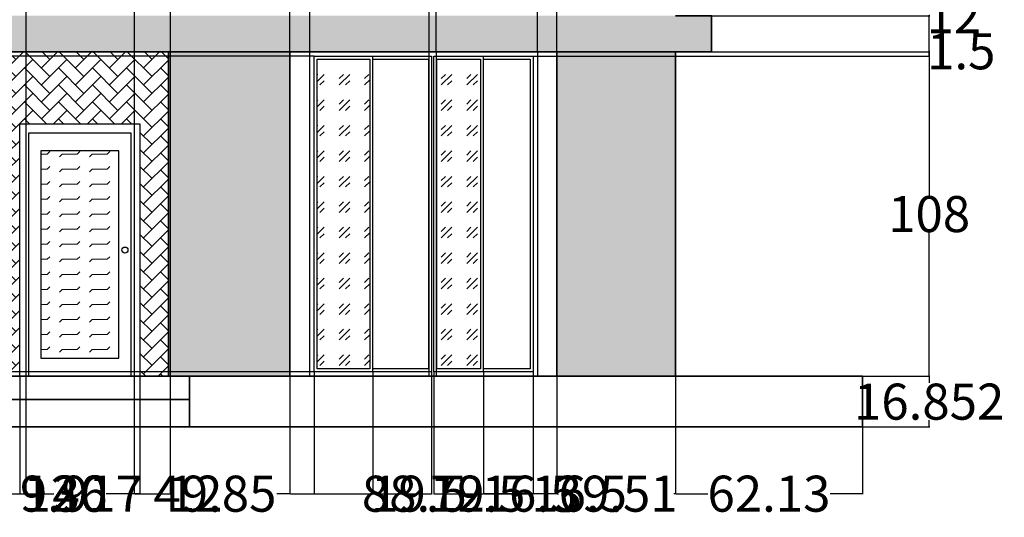
# Model space of a CAD drawing. Units: inches. Extents: x -73 to 458, y -161 to 332.
# Tile 2 of 6: x 106 to 433, y -161 to 5. Entities that reach past the tile are written whole.
import ezdxf

# ---------------------------------------------------------------- set-up
doc = ezdxf.new("R2010")
doc.units = ezdxf.units.IN
doc.header["$MEASUREMENT"] = 0
for name, color, linetype, lineweight in [('A-ANNO-DIMS', 2, 'Continuous', 18), ('A-DOOR', 4, 'Continuous', 25), ('A-ELEV', 7, 'Continuous', 35), ('A-ELEV-PATT', 8, 'Continuous', 13), ('A-GLAZ', 3, 'Continuous', 25), ('A-GLAZ-PATT', 8, 'Continuous', 13)]:
    doc.layers.add(name, color=color, linetype=linetype, lineweight=lineweight)
doc.styles.get("Standard").update_dxf_attribs({"font": 'arial.ttf'})
doc.dimstyles.get("Standard").update_dxf_attribs({"dimtxt": 12, "dimasz": 0.18, "dimexe": 0.18, "dimexo": 0.0625, "dimgap": 0.09, "dimtad": 0, "dimtih": 1, "dimtoh": 1, "dimdec": 0, "dimzin": 0, "dimdsep": 46, "dimlunit": 3, "dimtxsty": 'Standard', "dimcen": 0.09, "dimadec": 0, "dimazin": 0, "dimtfac": 1, "dimtdec": 0, "dimtofl": 0, "dimtmove": 0, "dimatfit": 3, "dimfxl": 1, "dimtolj": 1, "dimtzin": 0, "dimarcsym": 0})

# ---------------------------------------------------------------- blocks, each defined once
blk = doc.blocks.new('*U3')
blk.add_lwpolyline([(3.12, 0.01), (0.12, 0.01), (0.12, 84.01), (40.12, 84.01), (40.12, 0.01), (37.12, 0.01)])
for points in [[(37.12, 80.99), (37.12, 0.01), (3.12, 0.01), (3.12, 80.99)], [(33.12, 6.01), (33.12, 74.99), (7.12, 74.99), (7.12, 6.01)]]:
    blk.add_lwpolyline(points, close=True)
blk.add_circle((35.12, 42.01), 1)
blk = doc.blocks.new('*D11')
at = {"layer": 'A-ANNO-DIMS', "color": 0, "lineweight": -2, "transparency": 16777216}
for p, q in [((96, -114), (96, -153.17)), ((105.91, -113.98), (105.91, -153.17)), ((96.18, -152.99), (105.73, -152.99)), ((105.91, -152.99), (106.09, -152.99))]:
    blk.add_line(p, q, dxfattribs=at)
at = {"layer": 'A-ANNO-DIMS', "color": 0, "transparency": 16777216}
for points in [[(96.18, -152.96), (96.18, -153.02), (96, -152.99)], [(105.73, -152.96), (105.73, -153.02), (105.91, -152.99)]]:
    blk.add_solid(points, dxfattribs=at)
at = {"layer": 'Defpoints', "color": 0, "transparency": 16777216}
for p in [(96, -113.93), (105.91, -113.92), (105.91, -152.99)]:
    blk.add_point(p, dxfattribs=at)
at = {"layer": 'A-ANNO-DIMS', "color": 0, "transparency": 16777216, "insert": (126.43, -152.99), "char_height": 12, "attachment_point": 5}
blk.add_mtext('\\A1;9.917', dxfattribs=at)
blk = doc.blocks.new('*D12')
at = {"layer": 'A-ANNO-DIMS', "color": 0, "lineweight": -2, "transparency": 16777216}
for p, q in [((105.91, -113.98), (105.91, -153.17)), ((145.91, -113.98), (145.91, -153.17)), ((106.09, -152.99), (117.01, -152.99)), ((145.73, -152.99), (134.82, -152.99))]:
    blk.add_line(p, q, dxfattribs=at)
at = {"layer": 'A-ANNO-DIMS', "color": 0, "transparency": 16777216}
for points in [[(106.09, -152.96), (106.09, -153.02), (105.91, -152.99)], [(145.73, -152.96), (145.73, -153.02), (145.91, -152.99)]]:
    blk.add_solid(points, dxfattribs=at)
at = {"layer": 'Defpoints', "color": 0, "transparency": 16777216}
for p in [(105.91, -113.92), (145.91, -113.92), (145.91, -152.99)]:
    blk.add_point(p, dxfattribs=at)
at = {"layer": 'A-ANNO-DIMS', "color": 0, "transparency": 16777216, "insert": (125.91, -152.99), "char_height": 12, "attachment_point": 5}
blk.add_mtext('\\A1;40', dxfattribs=at)
blk = doc.blocks.new('*D13')
at = {"layer": 'A-ANNO-DIMS', "color": 0, "lineweight": -2, "transparency": 16777216}
for p, q in [((145.91, -113.98), (145.91, -153.17)), ((195.77, -114), (195.77, -153.17)), ((146.09, -152.99), (150.22, -152.99)), ((195.59, -152.99), (191.46, -152.99))]:
    blk.add_line(p, q, dxfattribs=at)
at = {"layer": 'A-ANNO-DIMS', "color": 0, "transparency": 16777216}
for points in [[(146.09, -152.96), (146.09, -153.02), (145.91, -152.99)], [(195.59, -152.96), (195.59, -153.02), (195.77, -152.99)]]:
    blk.add_solid(points, dxfattribs=at)
at = {"layer": 'Defpoints', "color": 0, "transparency": 16777216}
for p in [(145.91, -113.92), (195.77, -113.93), (195.77, -152.99)]:
    blk.add_point(p, dxfattribs=at)
at = {"layer": 'A-ANNO-DIMS', "color": 0, "transparency": 16777216, "insert": (170.84, -152.99), "char_height": 12, "attachment_point": 5}
blk.add_mtext('\\A1;49.85', dxfattribs=at)
blk = doc.blocks.new('*D14')
at = {"layer": 'A-ANNO-DIMS', "color": 0, "lineweight": -2, "transparency": 16777216}
for p, q in [((195.77, -114), (195.77, -153.17)), ((284.48, -114), (284.48, -153.17)), ((195.95, -152.99), (219.84, -152.99)), ((284.3, -152.99), (260.41, -152.99))]:
    blk.add_line(p, q, dxfattribs=at)
at = {"layer": 'A-ANNO-DIMS', "color": 0, "transparency": 16777216}
for points in [[(195.95, -152.96), (195.95, -153.02), (195.77, -152.99)], [(284.3, -152.96), (284.3, -153.02), (284.48, -152.99)]]:
    blk.add_solid(points, dxfattribs=at)
at = {"layer": 'Defpoints', "color": 0, "transparency": 16777216}
for p in [(195.77, -113.93), (284.48, -113.93), (284.48, -152.99)]:
    blk.add_point(p, dxfattribs=at)
at = {"layer": 'A-ANNO-DIMS', "color": 0, "transparency": 16777216, "insert": (240.13, -152.99), "char_height": 12, "attachment_point": 5}
blk.add_mtext('\\A1;88.72', dxfattribs=at)
blk = doc.blocks.new('*D15')
at = {"layer": 'A-ANNO-DIMS', "color": 0, "lineweight": -2, "transparency": 16777216}
for p, q in [((284.48, -114), (284.48, -153.17)), ((324, -114), (324, -153.17)), ((284.66, -152.99), (285.07, -152.99)), ((323.82, -152.99), (323.42, -152.99))]:
    blk.add_line(p, q, dxfattribs=at)
at = {"layer": 'A-ANNO-DIMS', "color": 0, "transparency": 16777216}
for points in [[(284.66, -152.96), (284.66, -153.02), (284.48, -152.99)], [(323.82, -152.96), (323.82, -153.02), (324, -152.99)]]:
    blk.add_solid(points, dxfattribs=at)
at = {"layer": 'Defpoints', "color": 0, "transparency": 16777216}
for p in [(284.48, -113.93), (324, -113.93), (324, -152.99)]:
    blk.add_point(p, dxfattribs=at)
at = {"layer": 'A-ANNO-DIMS', "color": 0, "transparency": 16777216, "insert": (304.24, -152.99), "char_height": 12, "attachment_point": 5}
blk.add_mtext('\\A1;39.51', dxfattribs=at)
blk = doc.blocks.new('*D16')
at = {"layer": 'A-ANNO-DIMS', "color": 0, "lineweight": -2, "transparency": 16777216}
for p, q in [((324, -114), (324, -153.17)), ((386.13, -130.85), (386.13, -153.17)), ((324.18, -152.99), (334.69, -152.99)), ((385.95, -152.99), (375.43, -152.99))]:
    blk.add_line(p, q, dxfattribs=at)
at = {"layer": 'A-ANNO-DIMS', "color": 0, "transparency": 16777216}
for points in [[(324.18, -152.96), (324.18, -153.02), (324, -152.99)], [(385.95, -152.96), (385.95, -153.02), (386.13, -152.99)]]:
    blk.add_solid(points, dxfattribs=at)
at = {"layer": 'Defpoints', "color": 0, "transparency": 16777216}
for p in [(324, -113.93), (386.13, -130.79), (386.13, -152.99)]:
    blk.add_point(p, dxfattribs=at)
at = {"layer": 'A-ANNO-DIMS', "color": 0, "transparency": 16777216, "insert": (355.06, -152.99), "char_height": 12, "attachment_point": 5}
blk.add_mtext('\\A1;62.13', dxfattribs=at)
blk = doc.blocks.new('*D17')
at = {"layer": 'A-ANNO-DIMS', "color": 0, "lineweight": -2, "transparency": 16777216}
for p, q in [((386.19, -113.93), (408.51, -113.93)), ((408.33, -114.11), (408.33, -116.14)), ((386.19, -130.79), (408.51, -130.79)), ((408.33, -130.61), (408.33, -128.58))]:
    blk.add_line(p, q, dxfattribs=at)
at = {"layer": 'A-ANNO-DIMS', "color": 0, "transparency": 16777216}
for points in [[(408.3, -114.11), (408.36, -114.11), (408.33, -113.93)], [(408.3, -130.61), (408.36, -130.61), (408.33, -130.79)]]:
    blk.add_solid(points, dxfattribs=at)
at = {"layer": 'Defpoints', "color": 0, "transparency": 16777216}
for p in [(386.13, -113.93), (408.33, -113.93), (386.13, -130.79)]:
    blk.add_point(p, dxfattribs=at)
at = {"layer": 'A-ANNO-DIMS', "color": 0, "transparency": 16777216, "insert": (408.33, -122.36), "char_height": 12, "attachment_point": 5}
blk.add_mtext('\\A1;16.852', dxfattribs=at)
blk = doc.blocks.new('*D18')
at = {"layer": 'A-ANNO-DIMS', "color": 0, "lineweight": -2, "transparency": 16777216}
for p, q in [((336.06, 6.07), (408.51, 6.07)), ((408.33, 6.07), (408.33, 6.25)), ((408.33, 6.25), (408.51, 6.25)), ((408.33, -5.75), (408.33, 5.89)), ((336.06, -5.93), (408.51, -5.93))]:
    blk.add_line(p, q, dxfattribs=at)
at = {"layer": 'A-ANNO-DIMS', "color": 0, "transparency": 16777216}
for points in [[(408.3, 5.89), (408.36, 5.89), (408.33, 6.07)], [(408.3, -5.75), (408.36, -5.75), (408.33, -5.93)]]:
    blk.add_solid(points, dxfattribs=at)
at = {"layer": 'Defpoints', "color": 0, "transparency": 16777216}
for p in [(336, 6.07), (408.33, 6.07), (336, -5.93)]:
    blk.add_point(p, dxfattribs=at)
at = {"layer": 'A-ANNO-DIMS', "color": 0, "transparency": 16777216, "insert": (416.56, 6.25), "char_height": 12, "attachment_point": 5}
blk.add_mtext('\\A1;12', dxfattribs=at)
blk = doc.blocks.new('*D19')
at = {"layer": 'A-ANNO-DIMS', "color": 0, "lineweight": -2, "transparency": 16777216}
for p, q in [((324.06, -5.93), (408.51, -5.93)), ((408.33, -6.11), (408.33, -53.72)), ((408.33, -113.75), (408.33, -66.15)), ((324.06, -113.93), (408.51, -113.93))]:
    blk.add_line(p, q, dxfattribs=at)
at = {"layer": 'A-ANNO-DIMS', "color": 0, "transparency": 16777216}
for points in [[(408.3, -6.11), (408.36, -6.11), (408.33, -5.93)], [(408.3, -113.75), (408.36, -113.75), (408.33, -113.93)]]:
    blk.add_solid(points, dxfattribs=at)
at = {"layer": 'Defpoints', "color": 0, "transparency": 16777216}
for p in [(324, -5.93), (408.33, -5.93), (324, -113.93)]:
    blk.add_point(p, dxfattribs=at)
at = {"layer": 'A-ANNO-DIMS', "color": 0, "transparency": 16777216, "insert": (408.33, -59.93), "char_height": 12, "attachment_point": 5}
blk.add_mtext('\\A1;108', dxfattribs=at)
blk = doc.blocks.new('*D36')
at = {"layer": 'A-ANNO-DIMS', "color": 0, "lineweight": -2, "transparency": 16777216}
for p, q in [((96, 53.96), (96, -153.17)), ((108, 53.96), (108, -153.17)), ((96.18, -152.99), (107.82, -152.99)), ((108, -152.99), (108.18, -152.99))]:
    blk.add_line(p, q, dxfattribs=at)
at = {"layer": 'A-ANNO-DIMS', "color": 0, "transparency": 16777216}
for points in [[(96.18, -152.96), (96.18, -153.02), (96, -152.99)], [(107.82, -152.96), (107.82, -153.02), (108, -152.99)]]:
    blk.add_solid(points, dxfattribs=at)
at = {"layer": 'Defpoints', "color": 0, "transparency": 16777216}
for p in [(96, 54.03), (108, 54.03), (108, -152.99)]:
    blk.add_point(p, dxfattribs=at)
at = {"layer": 'A-ANNO-DIMS', "color": 0, "transparency": 16777216, "insert": (116.24, -152.99), "char_height": 12, "attachment_point": 5}
blk.add_mtext('\\A1;12', dxfattribs=at)
blk = doc.blocks.new('*D37')
at = {"layer": 'A-ANNO-DIMS', "color": 0, "lineweight": -2, "transparency": 16777216}
for p, q in [((108, 53.96), (108, -153.17)), ((144, 53.96), (144, -153.17)), ((108.18, -152.99), (117.32, -152.99)), ((143.82, -152.99), (134.67, -152.99))]:
    blk.add_line(p, q, dxfattribs=at)
at = {"layer": 'A-ANNO-DIMS', "color": 0, "transparency": 16777216}
for points in [[(108.18, -152.96), (108.18, -153.02), (108, -152.99)], [(143.82, -152.96), (143.82, -153.02), (144, -152.99)]]:
    blk.add_solid(points, dxfattribs=at)
at = {"layer": 'Defpoints', "color": 0, "transparency": 16777216}
for p in [(108, 54.03), (144, 54.03), (144, -152.99)]:
    blk.add_point(p, dxfattribs=at)
at = {"layer": 'A-ANNO-DIMS', "color": 0, "transparency": 16777216, "insert": (126, -152.99), "char_height": 12, "attachment_point": 5}
blk.add_mtext('\\A1;36', dxfattribs=at)
blk = doc.blocks.new('*D38')
at = {"layer": 'A-ANNO-DIMS', "color": 0, "lineweight": -2, "transparency": 16777216}
for p, q in [((144, 53.96), (144, -153.17)), ((156, 53.96), (156, -153.17)), ((144.18, -152.99), (155.82, -152.99)), ((156, -152.99), (156.18, -152.99))]:
    blk.add_line(p, q, dxfattribs=at)
at = {"layer": 'A-ANNO-DIMS', "color": 0, "transparency": 16777216}
for points in [[(144.18, -152.96), (144.18, -153.02), (144, -152.99)], [(155.82, -152.96), (155.82, -153.02), (156, -152.99)]]:
    blk.add_solid(points, dxfattribs=at)
at = {"layer": 'Defpoints', "color": 0, "transparency": 16777216}
for p in [(144, 54.03), (156, 54.03), (156, -152.99)]:
    blk.add_point(p, dxfattribs=at)
at = {"layer": 'A-ANNO-DIMS', "color": 0, "transparency": 16777216, "insert": (164.24, -152.99), "char_height": 12, "attachment_point": 5}
blk.add_mtext('\\A1;12', dxfattribs=at)
blk = doc.blocks.new('*D71')
at = {"layer": 'A-ANNO-DIMS', "color": 0, "lineweight": -2, "transparency": 16777216}
for p, q in [((195.77, -5.87), (195.77, 324.4)), ((195.95, 324.22), (202.17, 324.22)), ((202.35, -5.87), (202.35, 324.4)), ((202.35, 324.22), (202.53, 324.22))]:
    blk.add_line(p, q, dxfattribs=at)
at = {"layer": 'A-ANNO-DIMS', "color": 0, "transparency": 16777216}
for points in [[(195.95, 324.25), (195.95, 324.19), (195.77, 324.22)], [(202.17, 324.25), (202.17, 324.19), (202.35, 324.22)]]:
    blk.add_solid(points, dxfattribs=at)
at = {"layer": 'Defpoints', "color": 0, "transparency": 16777216}
for p in [(202.35, 324.22), (195.77, -5.93), (202.35, -5.93)]:
    blk.add_point(p, dxfattribs=at)
at = {"layer": 'A-ANNO-DIMS', "color": 0, "transparency": 16777216, "insert": (222.95, 324.22), "char_height": 12, "attachment_point": 5}
blk.add_mtext('\\A1;6.585', dxfattribs=at)
blk = doc.blocks.new('*D72')
at = {"layer": 'A-ANNO-DIMS', "color": 0, "lineweight": -2, "transparency": 16777216}
for p, q in [((202.35, -5.87), (202.35, 324.4)), ((202.53, 324.22), (241.93, 324.22)), ((242.11, -5.87), (242.11, 324.4)), ((242.11, 324.22), (242.29, 324.22))]:
    blk.add_line(p, q, dxfattribs=at)
at = {"layer": 'A-ANNO-DIMS', "color": 0, "transparency": 16777216}
for points in [[(202.53, 324.25), (202.53, 324.19), (202.35, 324.22)], [(241.93, 324.25), (241.93, 324.19), (242.11, 324.22)]]:
    blk.add_solid(points, dxfattribs=at)
at = {"layer": 'Defpoints', "color": 0, "transparency": 16777216}
for p in [(242.11, 324.22), (202.35, -5.93), (242.11, -5.93)]:
    blk.add_point(p, dxfattribs=at)
at = {"layer": 'A-ANNO-DIMS', "color": 0, "transparency": 16777216, "insert": (262.62, 324.22), "char_height": 12, "attachment_point": 5}
blk.add_mtext('\\A1;39.76', dxfattribs=at)
blk = doc.blocks.new('*D73')
at = {"layer": 'A-ANNO-DIMS', "color": 0, "lineweight": -2, "transparency": 16777216}
for p, q in [((242.11, -5.87), (242.11, 324.4)), ((242.29, 324.22), (244.17, 324.22)), ((244.35, -5.87), (244.35, 324.4)), ((244.35, 324.22), (244.53, 324.22))]:
    blk.add_line(p, q, dxfattribs=at)
at = {"layer": 'A-ANNO-DIMS', "color": 0, "transparency": 16777216}
for points in [[(242.29, 324.25), (242.29, 324.19), (242.11, 324.22)], [(244.17, 324.25), (244.17, 324.19), (244.35, 324.22)]]:
    blk.add_solid(points, dxfattribs=at)
at = {"layer": 'Defpoints', "color": 0, "transparency": 16777216}
for p in [(244.35, 324.22), (242.11, -5.93), (244.35, -5.93)]:
    blk.add_point(p, dxfattribs=at)
at = {"layer": 'A-ANNO-DIMS', "color": 0, "transparency": 16777216, "insert": (264.95, 324.22), "char_height": 12, "attachment_point": 5}
blk.add_mtext('\\A1;2.244', dxfattribs=at)
blk = doc.blocks.new('*D74')
at = {"layer": 'A-ANNO-DIMS', "color": 0, "lineweight": -2, "transparency": 16777216}
for p, q in [((244.35, -5.87), (244.35, 324.4)), ((244.53, 324.22), (277.93, 324.22)), ((278.11, -5.87), (278.11, 324.4)), ((278.11, 324.22), (278.29, 324.22))]:
    blk.add_line(p, q, dxfattribs=at)
at = {"layer": 'A-ANNO-DIMS', "color": 0, "transparency": 16777216}
for points in [[(244.53, 324.25), (244.53, 324.19), (244.35, 324.22)], [(277.93, 324.25), (277.93, 324.19), (278.11, 324.22)]]:
    blk.add_solid(points, dxfattribs=at)
at = {"layer": 'Defpoints', "color": 0, "transparency": 16777216}
for p in [(278.11, 324.22), (244.35, -5.93), (278.11, -5.93)]:
    blk.add_point(p, dxfattribs=at)
at = {"layer": 'A-ANNO-DIMS', "color": 0, "transparency": 16777216, "insert": (303.28, 324.22), "char_height": 12, "attachment_point": 5}
blk.add_mtext('\\A1;33.756', dxfattribs=at)
blk = doc.blocks.new('*D75')
at = {"layer": 'A-ANNO-DIMS', "color": 0, "lineweight": -2, "transparency": 16777216}
for p, q in [((278.11, -5.87), (278.11, 324.4)), ((278.29, 324.22), (284.3, 324.22)), ((284.48, -5.87), (284.48, 324.4)), ((284.48, 324.22), (284.66, 324.22))]:
    blk.add_line(p, q, dxfattribs=at)
at = {"layer": 'A-ANNO-DIMS', "color": 0, "transparency": 16777216}
for points in [[(278.29, 324.25), (278.29, 324.19), (278.11, 324.22)], [(284.3, 324.25), (284.3, 324.19), (284.48, 324.22)]]:
    blk.add_solid(points, dxfattribs=at)
at = {"layer": 'Defpoints', "color": 0, "transparency": 16777216}
for p in [(284.48, 324.22), (278.11, -5.93), (284.48, -5.93)]:
    blk.add_point(p, dxfattribs=at)
at = {"layer": 'A-ANNO-DIMS', "color": 0, "transparency": 16777216, "insert": (305.03, 324.22), "char_height": 12, "attachment_point": 5}
blk.add_mtext('\\A1;6.377', dxfattribs=at)
blk = doc.blocks.new('*D76')
at = {"layer": 'A-ANNO-DIMS', "color": 0, "lineweight": -2, "transparency": 16777216}
for p, q in [((278.17, -5.93), (408.51, -5.93)), ((408.33, -5.93), (408.33, -5.75)), ((408.33, -5.75), (408.51, -5.75)), ((408.33, -7.25), (408.33, -6.11)), ((276.67, -7.43), (408.51, -7.43))]:
    blk.add_line(p, q, dxfattribs=at)
at = {"layer": 'A-ANNO-DIMS', "color": 0, "transparency": 16777216}
for points in [[(408.3, -6.11), (408.36, -6.11), (408.33, -5.93)], [(408.3, -7.25), (408.36, -7.25), (408.33, -7.43)]]:
    blk.add_solid(points, dxfattribs=at)
at = {"layer": 'Defpoints', "color": 0, "transparency": 16777216}
for p in [(278.11, -5.93), (408.33, -5.93), (276.61, -7.43)]:
    blk.add_point(p, dxfattribs=at)
at = {"layer": 'A-ANNO-DIMS', "color": 0, "transparency": 16777216, "insert": (419, -5.75), "char_height": 12, "attachment_point": 5}
blk.add_mtext('\\A1;1.5', dxfattribs=at)
blk = doc.blocks.new('*D77')
at = {"layer": 'A-ANNO-DIMS', "color": 0, "lineweight": -2, "transparency": 16777216}
for p, q in [((203.85, -112.5), (203.85, -153.17)), ((223.35, -112.5), (223.35, -153.17)), ((204.03, -152.99), (223.17, -152.99)), ((223.35, -152.99), (223.53, -152.99))]:
    blk.add_line(p, q, dxfattribs=at)
at = {"layer": 'A-ANNO-DIMS', "color": 0, "transparency": 16777216}
for points in [[(204.03, -152.96), (204.03, -153.02), (203.85, -152.99)], [(223.17, -152.96), (223.17, -153.02), (223.35, -152.99)]]:
    blk.add_solid(points, dxfattribs=at)
at = {"layer": 'Defpoints', "color": 0, "transparency": 16777216}
for p in [(203.85, -112.43), (223.35, -112.43), (223.35, -152.99)]:
    blk.add_point(p, dxfattribs=at)
at = {"layer": 'A-ANNO-DIMS', "color": 0, "transparency": 16777216, "insert": (238.69, -152.99), "char_height": 12, "attachment_point": 5}
blk.add_mtext('\\A1;19.5', dxfattribs=at)
blk = doc.blocks.new('*D78')
at = {"layer": 'A-ANNO-DIMS', "color": 0, "lineweight": -2, "transparency": 16777216}
for p, q in [((223.35, -112.5), (223.35, -153.17)), ((242.85, -112.5), (242.85, -153.17)), ((223.53, -152.99), (242.67, -152.99)), ((242.85, -152.99), (243.03, -152.99))]:
    blk.add_line(p, q, dxfattribs=at)
at = {"layer": 'A-ANNO-DIMS', "color": 0, "transparency": 16777216}
for points in [[(223.53, -152.96), (223.53, -153.02), (223.35, -152.99)], [(242.67, -152.96), (242.67, -153.02), (242.85, -152.99)]]:
    blk.add_solid(points, dxfattribs=at)
at = {"layer": 'Defpoints', "color": 0, "transparency": 16777216}
for p in [(223.35, -112.43), (242.85, -112.43), (242.85, -152.99)]:
    blk.add_point(p, dxfattribs=at)
at = {"layer": 'A-ANNO-DIMS', "color": 0, "transparency": 16777216, "insert": (258.19, -152.99), "char_height": 12, "attachment_point": 5}
blk.add_mtext('\\A1;19.5', dxfattribs=at)
blk = doc.blocks.new('*D79')
at = {"layer": 'A-ANNO-DIMS', "color": 0, "lineweight": -2, "transparency": 16777216}
for p, q in [((243.61, -112.5), (243.61, -153.17)), ((260.11, -112.5), (260.11, -153.17)), ((243.79, -152.99), (259.93, -152.99)), ((260.11, -152.99), (260.29, -152.99))]:
    blk.add_line(p, q, dxfattribs=at)
at = {"layer": 'A-ANNO-DIMS', "color": 0, "transparency": 16777216}
for points in [[(243.79, -152.96), (243.79, -153.02), (243.61, -152.99)], [(259.93, -152.96), (259.93, -153.02), (260.11, -152.99)]]:
    blk.add_solid(points, dxfattribs=at)
at = {"layer": 'Defpoints', "color": 0, "transparency": 16777216}
for p in [(243.61, -112.43), (260.11, -112.43), (260.11, -152.99)]:
    blk.add_point(p, dxfattribs=at)
at = {"layer": 'A-ANNO-DIMS', "color": 0, "transparency": 16777216, "insert": (275.44, -152.99), "char_height": 12, "attachment_point": 5}
blk.add_mtext('\\A1;16.5', dxfattribs=at)
blk = doc.blocks.new('*D80')
at = {"layer": 'A-ANNO-DIMS', "color": 0, "lineweight": -2, "transparency": 16777216}
for p, q in [((260.11, -112.5), (260.11, -153.17)), ((276.61, -112.5), (276.61, -153.17)), ((260.29, -152.99), (276.43, -152.99)), ((276.61, -152.99), (276.79, -152.99))]:
    blk.add_line(p, q, dxfattribs=at)
at = {"layer": 'A-ANNO-DIMS', "color": 0, "transparency": 16777216}
for points in [[(260.29, -152.96), (260.29, -153.02), (260.11, -152.99)], [(276.43, -152.96), (276.43, -153.02), (276.61, -152.99)]]:
    blk.add_solid(points, dxfattribs=at)
at = {"layer": 'Defpoints', "color": 0, "transparency": 16777216}
for p in [(260.11, -112.43), (276.61, -112.43), (276.61, -152.99)]:
    blk.add_point(p, dxfattribs=at)
at = {"layer": 'A-ANNO-DIMS', "color": 0, "transparency": 16777216, "insert": (291.94, -152.99), "char_height": 12, "attachment_point": 5}
blk.add_mtext('\\A1;16.5', dxfattribs=at)
blk = doc.blocks.new('*D81')
at = {"layer": 'A-ANNO-DIMS', "color": 0, "lineweight": -2, "transparency": 16777216}
for p, q in [((203.79, -7.43), (-41.78, -7.43)), ((-41.6, -7.61), (-41.6, -53.72)), ((-41.6, -112.25), (-41.6, -66.15)), ((203.79, -112.43), (-41.78, -112.43))]:
    blk.add_line(p, q, dxfattribs=at)
at = {"layer": 'A-ANNO-DIMS', "color": 0, "transparency": 16777216}
for points in [[(-41.63, -7.61), (-41.57, -7.61), (-41.6, -7.43)], [(-41.63, -112.25), (-41.57, -112.25), (-41.6, -112.43)]]:
    blk.add_solid(points, dxfattribs=at)
at = {"layer": 'Defpoints', "color": 0, "transparency": 16777216}
for p in [(-41.6, -7.43), (203.85, -7.43), (203.85, -112.43)]:
    blk.add_point(p, dxfattribs=at)
at = {"layer": 'A-ANNO-DIMS', "color": 0, "transparency": 16777216, "insert": (-41.6, -59.93), "char_height": 12, "attachment_point": 5}
blk.add_mtext('\\A1;105', dxfattribs=at)

msp = doc.modelspace()

# ---------------------------------------------------------------- hatches: boundary and pattern name
at = {"layer": 'A-ELEV-PATT'}
h = msp.add_hatch(color=256, dxfattribs=at)
h.dxf.hatch_style = 1
h.paths.add_polyline_path([(167.9979, 302.0202), (155.9979, 302.0202), (95.9979, 302.0202), (23.9979, 302.0202), (23.9979, -113.9335), (33.9979, -113.9335), (33.9979, 292.0202), (95.9979, 292.0202), (157.9979, 292.0202), (157.9979, 260.2059), (167.9979, 260.2059), (167.9979, 290.0202)])
h.paths.add_polyline_path([(335.9979, 242.2059), (323.9979, 242.2059), (95.9979, 242.2059), (95.9979, 234.0665), (95.9979, 230.2059), (323.9979, 230.2059), (335.9979, 230.2059)])
h.paths.add_polyline_path([(335.9979, 126.0665), (323.9979, 126.0665), (173.9979, 126.0665), (173.9979, 114.0665), (323.9979, 114.0665), (335.9979, 114.0665)])
h.paths.add_polyline_path([(335.9979, 6.0665), (323.9979, 6.0665), (95.9979, 6.0665), (95.9979, -5.9335), (323.9979, -5.9335), (335.9979, -5.9335)])
h = msp.add_hatch(color=256, dxfattribs=at)
h.dxf.hatch_style = 1
h.paths.add_polyline_path([(195.7666, -5.9335), (155.3839, -5.9335), (155.3839, -113.9335), (195.7666, -113.9335)])
h.paths.add_polyline_path([(323.9979, -5.9335), (284.4845, -5.9335), (284.4845, -113.9335), (323.9979, -113.9335)])
h.paths.add_polyline_path([(203.9979, 114.0665), (173.9979, 114.0665), (173.9979, 144.0665), (203.9979, 144.0665), (203.9979, 230.2059), (155.9979, 230.2059), (155.9979, 24.0665), (203.9979, 24.0665)])
h = msp.add_hatch(dxfattribs=at)
h.set_pattern_fill('FLEX', color=256, scale=20)
h.paths.add_polyline_path([(241.805, 219.0563), (215.805, 219.0563), (215.805, 150.0793), (241.805, 150.0793)])
h.paths.add_polyline_path([(241.805, 99.0563), (215.805, 99.0563), (215.805, 30.0793), (241.805, 30.0793)])
h.paths.add_polyline_path([(138.915, -38.9437), (112.915, -38.9437), (112.915, -107.9207), (138.915, -107.9207)])
h = msp.add_hatch(dxfattribs=at)
h.set_pattern_fill('AR-HBONE', color=256)
h.paths.add_polyline_path([(155.3839, -5.9335), (95.9979, -5.9335), (95.9979, -113.9335), (105.915, -113.9335), (105.915, -29.9207), (145.915, -29.9207), (145.915, -113.9335), (155.3839, -113.9335)])

# ---------------------------------------------------------------- linework, layer by layer
at = {"layer": 'A-ELEV'}
for p, q in [((95.9979, -5.9335), (323.9979, -5.9335)), ((23.9979, -113.9335), (323.9979, -113.9335))]:
    msp.add_line(p, q, dxfattribs=at)
msp.add_lwpolyline([(323.9979, 6.0665), (335.9979, 6.0665), (335.9979, -5.9335), (323.9979, -5.9335)], dxfattribs=at)
for points in [[(155.3839, -113.9335), (195.7666, -113.9335), (195.7666, -5.9335), (155.3839, -5.9335)], [(284.4845, -113.9335), (323.9979, -113.9335), (323.9979, -5.9335), (284.4845, -5.9335)], [(386.126, -113.9335), (-19.4031, -113.9335), (-19.4031, -130.7857), (386.126, -130.7857)], [(95.9979, -113.9335), (162.3543, -113.9335), (162.3543, -121.6608), (95.9979, -121.6608)], [(95.9979, -121.6608), (162.3543, -121.6608), (162.3543, -130.7857), (95.9979, -130.7857)]]:
    msp.add_lwpolyline(points, close=True, dxfattribs=at)
at = {"layer": 'A-GLAZ'}
for p, q in [((203.8513, -112.4335), (203.8513, -7.4335)), ((203.8513, -7.4335), (223.3513, -7.4335)), ((223.3513, -112.4335), (223.3513, -7.4335)), ((223.3513, -7.4335), (242.8513, -7.4335)), ((242.8513, -7.4335), (242.8513, -112.4335)), ((243.6074, -112.4335), (243.6074, -7.4335)), ((243.6074, -7.4335), (260.1074, -7.4335)), ((260.1074, -112.4335), (260.1074, -7.4335)), ((260.1074, -7.4335), (276.6074, -7.4335)), ((276.6074, -7.4335), (276.6074, -112.4335)), ((223.3513, -112.4335), (203.8513, -112.4335)), ((242.8513, -112.4335), (223.3513, -112.4335)), ((260.1074, -112.4335), (243.6074, -112.4335)), ((276.6074, -112.4335), (260.1074, -112.4335))]:
    msp.add_line(p, q, dxfattribs=at)
for points in [[(202.3513, -113.9335), (202.3513, -5.9335), (244.3513, -5.9335), (244.3513, -113.9335)], [(242.1074, -113.9335), (242.1074, -5.9335), (278.1074, -5.9335), (278.1074, -113.9335)]]:
    msp.add_lwpolyline(points, close=True, dxfattribs=at)
for points in [[(222.3513, -8.4334), (222.3513, -111.4335), (204.8513, -111.4335), (204.8513, -8.4335), (222.3513, -8.4335)], [(223.3513, -8.4335), (241.8513, -8.4335), (241.8513, -111.4335), (223.3513, -111.4335)], [(259.1074, -8.4334), (259.1074, -111.4335), (244.6074, -111.4335), (244.6074, -8.4335), (259.1074, -8.4335)], [(260.1074, -8.4335), (275.6074, -8.4335), (275.6074, -111.4335), (260.1074, -111.4335)]]:
    msp.add_lwpolyline(points, dxfattribs=at)
at = {"layer": 'A-GLAZ-PATT'}
for p, q in [((205.7681, -8.4853), (205.8199, -8.4335)), ((212.132, -8.4853), (212.1838, -8.4335)), ((214.2534, -8.4853), (214.3052, -8.4335)), ((220.6173, -8.4853), (220.6691, -8.4335)), ((246.0732, -8.4853), (246.125, -8.4335)), ((248.1945, -8.4853), (248.2463, -8.4335)), ((254.5584, -8.4853), (254.6103, -8.4335)), ((256.6798, -8.4853), (256.7316, -8.4335)), ((204.8513, -15.766), (207.1823, -13.435)), ((204.8513, -13.6447), (205.061, -13.435)), ((205.7681, -16.9706), (207.1823, -15.5563)), ((212.132, -16.9706), (215.6676, -13.435)), ((212.132, -14.8492), (213.5462, -13.435)), ((214.2534, -16.9706), (215.6676, -15.5563)), ((220.6173, -14.8492), (222.0315, -13.435)), ((220.6173, -16.9706), (222.3513, -15.2366)), ((246.0732, -16.9706), (249.6087, -13.435)), ((246.0732, -14.8492), (247.4874, -13.435)), ((248.1945, -16.9706), (249.6087, -15.5563)), ((254.5584, -16.9706), (258.094, -13.435)), ((254.5584, -14.8492), (255.9727, -13.435)), ((256.6798, -16.9706), (258.094, -15.5563)), ((204.8513, -24.2513), (207.1823, -21.9203)), ((204.8513, -22.13), (205.061, -21.9203)), ((212.132, -25.4558), (215.6676, -21.9203)), ((212.132, -23.3345), (213.5462, -21.9203)), ((220.6173, -23.3345), (222.0315, -21.9203)), ((246.0732, -25.4558), (249.6087, -21.9203)), ((246.0732, -23.3345), (247.4874, -21.9203)), ((254.5584, -25.4558), (258.094, -21.9203)), ((254.5584, -23.3345), (255.9727, -21.9203)), ((205.7681, -25.4558), (207.1823, -24.0416)), ((214.2534, -25.4558), (215.6676, -24.0416)), ((220.6173, -25.4558), (222.3513, -23.7219)), ((248.1945, -25.4558), (249.6087, -24.0416)), ((256.6798, -25.4558), (258.094, -24.0416)), ((204.8513, -32.7366), (207.1823, -30.4056)), ((204.8513, -30.6153), (205.061, -30.4056)), ((205.7681, -33.9411), (207.1823, -32.5269)), ((212.132, -33.9411), (215.6676, -30.4056)), ((212.132, -31.8198), (213.5462, -30.4056)), ((214.2534, -33.9411), (215.6676, -32.5269)), ((220.6173, -31.8198), (222.0315, -30.4056)), ((220.6173, -33.9411), (222.3513, -32.2071)), ((246.0732, -33.9411), (249.6087, -30.4056)), ((246.0732, -31.8198), (247.4874, -30.4056)), ((248.1945, -33.9411), (249.6087, -32.5269)), ((254.5584, -33.9411), (258.094, -30.4056)), ((254.5584, -31.8198), (255.9727, -30.4056)), ((256.6798, -33.9411), (258.094, -32.5269)), ((204.8513, -41.2219), (207.1823, -38.8909)), ((204.8513, -39.1005), (205.061, -38.8909)), ((212.132, -42.4264), (215.6676, -38.8909)), ((212.132, -40.3051), (213.5462, -38.8909)), ((220.6173, -40.3051), (222.0315, -38.8909)), ((246.0732, -42.4264), (249.6087, -38.8909)), ((246.0732, -40.3051), (247.4874, -38.8909)), ((254.5584, -42.4264), (258.094, -38.8909)), ((254.5584, -40.3051), (255.9727, -38.8909)), ((205.7681, -42.4264), (207.1823, -41.0122)), ((214.2534, -42.4264), (215.6676, -41.0122)), ((220.6173, -42.4264), (222.3513, -40.6924)), ((248.1945, -42.4264), (249.6087, -41.0122)), ((256.6798, -42.4264), (258.094, -41.0122)), ((204.8513, -49.7071), (207.1823, -47.3762)), ((204.8513, -47.5858), (205.061, -47.3762)), ((212.132, -50.9117), (215.6676, -47.3762)), ((212.132, -48.7904), (213.5462, -47.3762)), ((220.6173, -48.7904), (222.0315, -47.3762)), ((246.0732, -50.9117), (249.6087, -47.3762)), ((246.0732, -48.7904), (247.4874, -47.3762)), ((254.5584, -50.9117), (258.094, -47.3762)), ((254.5584, -48.7904), (255.9727, -47.3762)), ((205.7681, -50.9117), (207.1823, -49.4975)), ((214.2534, -50.9117), (215.6676, -49.4975)), ((220.6173, -50.9117), (222.3513, -49.1777)), ((248.1945, -50.9117), (249.6087, -49.4975)), ((256.6798, -50.9117), (258.094, -49.4975)), ((204.8513, -58.1924), (207.1823, -55.8614)), ((204.8513, -56.0711), (205.061, -55.8614)), ((205.7681, -59.397), (207.1823, -57.9828)), ((212.132, -59.397), (215.6676, -55.8614)), ((212.132, -57.2756), (213.5462, -55.8614)), ((214.2534, -59.397), (215.6676, -57.9828)), ((220.6173, -57.2756), (222.0315, -55.8614)), ((220.6173, -59.397), (222.3513, -57.663)), ((246.0732, -59.397), (249.6087, -55.8614)), ((246.0732, -57.2756), (247.4874, -55.8614)), ((248.1945, -59.397), (249.6087, -57.9828)), ((254.5584, -59.397), (258.094, -55.8614)), ((254.5584, -57.2756), (255.9727, -55.8614)), ((256.6798, -59.397), (258.094, -57.9828)), ((204.8513, -66.6777), (207.1823, -64.3467)), ((204.8513, -64.5564), (205.061, -64.3467)), ((212.132, -67.8823), (215.6676, -64.3467)), ((212.132, -65.7609), (213.5462, -64.3467)), ((220.6173, -65.7609), (222.0315, -64.3467)), ((246.0732, -67.8823), (249.6087, -64.3467)), ((246.0732, -65.7609), (247.4874, -64.3467)), ((254.5584, -67.8823), (258.094, -64.3467)), ((254.5584, -65.7609), (255.9727, -64.3467)), ((205.7681, -67.8823), (207.1823, -66.468)), ((214.2534, -67.8823), (215.6676, -66.468)), ((220.6173, -67.8823), (222.3513, -66.1483)), ((248.1945, -67.8823), (249.6087, -66.468)), ((256.6798, -67.8823), (258.094, -66.468)), ((204.8513, -75.163), (207.1823, -72.832)), ((204.8513, -73.0417), (205.061, -72.832)), ((205.7681, -76.3675), (207.1823, -74.9533)), ((212.132, -76.3675), (215.6676, -72.832)), ((212.132, -74.2462), (213.5462, -72.832)), ((214.2534, -76.3675), (215.6676, -74.9533)), ((220.6173, -74.2462), (222.0315, -72.832)), ((220.6173, -76.3675), (222.3513, -74.6336)), ((246.0732, -76.3675), (249.6087, -72.832)), ((246.0732, -74.2462), (247.4874, -72.832)), ((248.1945, -76.3675), (249.6087, -74.9533)), ((254.5584, -76.3675), (258.094, -72.832)), ((254.5584, -74.2462), (255.9727, -72.832)), ((256.6798, -76.3675), (258.094, -74.9533)), ((204.8513, -83.6483), (207.1823, -81.3173)), ((204.8513, -81.527), (205.061, -81.3173)), ((212.132, -84.8528), (215.6676, -81.3173)), ((212.132, -82.7315), (213.5462, -81.3173)), ((220.6173, -82.7315), (222.0315, -81.3173)), ((246.0732, -84.8528), (249.6087, -81.3173)), ((246.0732, -82.7315), (247.4874, -81.3173)), ((254.5584, -84.8528), (258.094, -81.3173)), ((254.5584, -82.7315), (255.9727, -81.3173)), ((205.7681, -84.8528), (207.1823, -83.4386)), ((214.2534, -84.8528), (215.6676, -83.4386)), ((220.6173, -84.8528), (222.3513, -83.1188)), ((248.1945, -84.8528), (249.6087, -83.4386)), ((256.6798, -84.8528), (258.094, -83.4386)), ((204.8513, -92.1336), (207.1823, -89.8026)), ((204.8513, -90.0122), (205.061, -89.8026)), ((212.132, -93.3381), (215.6676, -89.8026)), ((212.132, -91.2168), (213.5462, -89.8026)), ((220.6173, -91.2168), (222.0315, -89.8026)), ((220.6173, -93.3381), (222.3513, -91.6041)), ((246.0732, -93.3381), (249.6087, -89.8026)), ((246.0732, -91.2168), (247.4874, -89.8026)), ((254.5584, -93.3381), (258.094, -89.8026)), ((254.5584, -91.2168), (255.9727, -89.8026)), ((205.7681, -93.3381), (207.1823, -91.9239)), ((214.2534, -93.3381), (215.6676, -91.9239)), ((248.1945, -93.3381), (249.6087, -91.9239)), ((256.6798, -93.3381), (258.094, -91.9239)), ((204.8513, -100.6188), (207.1823, -98.2878)), ((204.8513, -98.4975), (205.061, -98.2878)), ((205.7681, -101.8234), (207.1823, -100.4092)), ((212.132, -101.8234), (215.6676, -98.2878)), ((212.132, -99.7021), (213.5462, -98.2878)), ((214.2534, -101.8234), (215.6676, -100.4092)), ((220.6173, -99.7021), (222.0315, -98.2878)), ((220.6173, -101.8234), (222.3513, -100.0894)), ((246.0732, -101.8234), (249.6087, -98.2878)), ((246.0732, -99.7021), (247.4874, -98.2878)), ((248.1945, -101.8234), (249.6087, -100.4092)), ((254.5584, -101.8234), (258.094, -98.2878)), ((254.5584, -99.7021), (255.9727, -98.2878)), ((256.6798, -101.8234), (258.094, -100.4092)), ((204.8513, -109.1041), (207.1823, -106.7731)), ((204.8513, -106.9828), (205.061, -106.7731)), ((212.132, -110.3087), (215.6676, -106.7731)), ((212.132, -108.1873), (213.5462, -106.7731)), ((220.6173, -108.1873), (222.0315, -106.7731)), ((246.0732, -110.3087), (249.6087, -106.7731)), ((246.0732, -108.1873), (247.4874, -106.7731)), ((254.5584, -110.3087), (258.094, -106.7731)), ((254.5584, -108.1873), (255.9727, -106.7731)), ((205.7681, -110.3087), (207.1823, -108.8944)), ((214.2534, -110.3087), (215.6676, -108.8944)), ((220.6173, -110.3087), (222.3513, -108.5747)), ((248.1945, -110.3087), (249.6087, -108.8944)), ((256.6798, -110.3087), (258.094, -108.8944))]:
    msp.add_line(p, q, dxfattribs=at)

# ---------------------------------------------------------------- block references
at = {"layer": 'A-DOOR'}
msp.add_blockref('*U3', (105.7912, -113.9335), dxfattribs=at)

# ---------------------------------------------------------------- dimensions: what is measured, and where the dimension line sits
at = {"layer": 'A-ANNO-DIMS'}
for base, p1, p2, override, picture, middle in [((202.3513, 324.2202), (195.7666, -5.9335), (202.3513, -5.9335), {"dimdec": 3, "dimlfac": 1, "dimrnd": 0, "dimzin": 0, "dimdsep": 46, "dimlunit": 2}, '*D71', (222.946, 324.2202)), ((242.1074, 324.2202), (202.3513, -5.9335), (242.1074, -5.9335), {"dimdec": 2, "dimlfac": 1, "dimrnd": 0, "dimzin": 0, "dimdsep": 46, "dimlunit": 2}, '*D72', (262.6161, 324.2202)), ((244.3513, 324.2202), (242.1074, -5.9335), (244.3513, -5.9335), {"dimdec": 3, "dimlfac": 1, "dimrnd": 0, "dimzin": 0, "dimdsep": 46, "dimlunit": 2}, '*D73', (264.946, 324.2202)), ((278.1074, 324.2202), (244.3513, -5.9335), (278.1074, -5.9335), {"dimdec": 3, "dimlfac": 1, "dimrnd": 0, "dimzin": 0, "dimdsep": 46, "dimlunit": 2}, '*D74', (303.2778, 324.2202)), ((284.4845, 324.2202), (278.1074, -5.9335), (284.4845, -5.9335), {"dimdec": 3, "dimlfac": 1, "dimrnd": 0, "dimzin": 0, "dimdsep": 46, "dimlunit": 2}, '*D75', (305.0342, 324.2202)), ((107.9979, -152.9857), (95.9979, 54.0267), (107.9979, 54.0267), {"dimdec": 0, "dimlfac": 1, "dimrnd": 0, "dimzin": 0, "dimdsep": 46, "dimlunit": 2}, '*D36', (116.2365, -152.9857)), ((143.9979, -152.9857), (107.9979, 54.0267), (143.9979, 54.0267), {"dimdec": 0, "dimlfac": 1, "dimrnd": 0, "dimzin": 0, "dimdsep": 46, "dimlunit": 2}, '*D37', (125.9979, -152.9857)), ((155.9979, -152.9857), (143.9979, 54.0267), (155.9979, 54.0267), {"dimdec": 0, "dimlfac": 1, "dimrnd": 0, "dimzin": 0, "dimdsep": 46, "dimlunit": 2}, '*D38', (164.2365, -152.9857)), ((105.915, -152.9857), (95.9979, -113.9335), (105.915, -113.9207), {"dimdec": 3, "dimlfac": 1, "dimrnd": 0, "dimzin": 0, "dimdsep": 46, "dimlunit": 2}, '*D11', (126.4319, -152.9857)), ((145.915, -152.9857), (105.915, -113.9207), (145.915, -113.9207), {"dimdec": 0, "dimlfac": 1, "dimrnd": 0, "dimzin": 0, "dimdsep": 46, "dimlunit": 2}, '*D12', (125.915, -152.9857)), ((195.7666, -152.9857), (145.915, -113.9207), (195.7666, -113.9335), {"dimdec": 2, "dimlfac": 1, "dimrnd": 0, "dimzin": 0, "dimdsep": 46, "dimlunit": 2}, '*D13', (170.8408, -152.9857)), ((284.4845, -152.9857), (195.7666, -113.9335), (284.4845, -113.9335), {"dimdec": 2, "dimlfac": 1, "dimrnd": 0, "dimzin": 0, "dimdsep": 46, "dimlunit": 2}, '*D14', (240.1255, -152.9857)), ((223.3513, -152.9857), (203.8513, -112.4335), (223.3513, -112.4335), {"dimdec": 1, "dimlfac": 1, "dimrnd": 0, "dimzin": 0, "dimdsep": 46, "dimlunit": 2}, '*D77', (238.6868, -152.9857)), ((242.8513, -152.9857), (223.3513, -112.4335), (242.8513, -112.4335), {"dimdec": 1, "dimlfac": 1, "dimrnd": 0, "dimzin": 0, "dimdsep": 46, "dimlunit": 2}, '*D78', (258.1868, -152.9857)), ((260.1074, -152.9857), (243.6074, -112.4335), (260.1074, -112.4335), {"dimdec": 1, "dimlfac": 1, "dimrnd": 0, "dimzin": 0, "dimdsep": 46, "dimlunit": 2}, '*D79', (275.4429, -152.9857)), ((276.6074, -152.9857), (260.1074, -112.4335), (276.6074, -112.4335), {"dimdec": 1, "dimlfac": 1, "dimrnd": 0, "dimzin": 0, "dimdsep": 46, "dimlunit": 2}, '*D80', (291.9429, -152.9857)), ((323.9979, -152.9857), (284.4845, -113.9335), (323.9979, -113.9335), {"dimdec": 2, "dimlfac": 1, "dimrnd": 0, "dimzin": 0, "dimdsep": 46, "dimlunit": 2}, '*D15', (304.2412, -152.9857)), ((386.126, -152.9857), (323.9979, -113.9335), (386.126, -130.7857), {"dimdec": 2, "dimlfac": 1, "dimrnd": 0, "dimzin": 0, "dimdsep": 46, "dimlunit": 2}, '*D16', (355.0619, -152.9857))]:
    dim = msp.add_linear_dim(base=base, p1=p1, p2=p2, dimstyle='Standard', override=override, dxfattribs=at)
    dim.commit()
    dim.dimension.update_dxf_attribs({"geometry": picture, "text_midpoint": middle})
for base, p1, p2, override, picture, middle in [((408.326, 6.0665), (335.9979, -5.9335), (335.9979, 6.0665), {"dimdec": 0, "dimlfac": 1, "dimrnd": 0, "dimzin": 0, "dimdsep": 46, "dimlunit": 2}, '*D18', (416.5646, 6.2465)), ((408.326, -5.9335), (276.6074, -7.4335), (278.1074, -5.9335), {"dimdec": 1, "dimlfac": 1, "dimrnd": 0, "dimzin": 0, "dimdsep": 46, "dimlunit": 2}, '*D76', (418.9998, -5.7535)), ((408.326, -5.9335), (323.9979, -113.9335), (323.9979, -5.9335), {"dimdec": 0, "dimlfac": 1, "dimrnd": 0, "dimzin": 0, "dimdsep": 46, "dimlunit": 2}, '*D19', (408.326, -59.9335)), ((-41.6031, -7.4335), (203.8513, -112.4335), (203.8513, -7.4335), {"dimdec": 0, "dimlfac": 1, "dimrnd": 0, "dimzin": 0, "dimdsep": 46, "dimlunit": 2}, '*D81', (-41.6031, -59.9335)), ((408.326, -113.9335), (386.126, -130.7857), (386.126, -113.9335), {"dimdec": 3, "dimlfac": 1, "dimrnd": 0, "dimzin": 0, "dimdsep": 46, "dimlunit": 2}, '*D17', (408.326, -122.3596))]:
    dim = msp.add_linear_dim(base=base, p1=p1, p2=p2, angle=90, dimstyle='Standard', override=override, dxfattribs=at)
    dim.commit()
    dim.dimension.update_dxf_attribs({"geometry": picture, "text_midpoint": middle})

doc.saveas('drawing.dxf')
